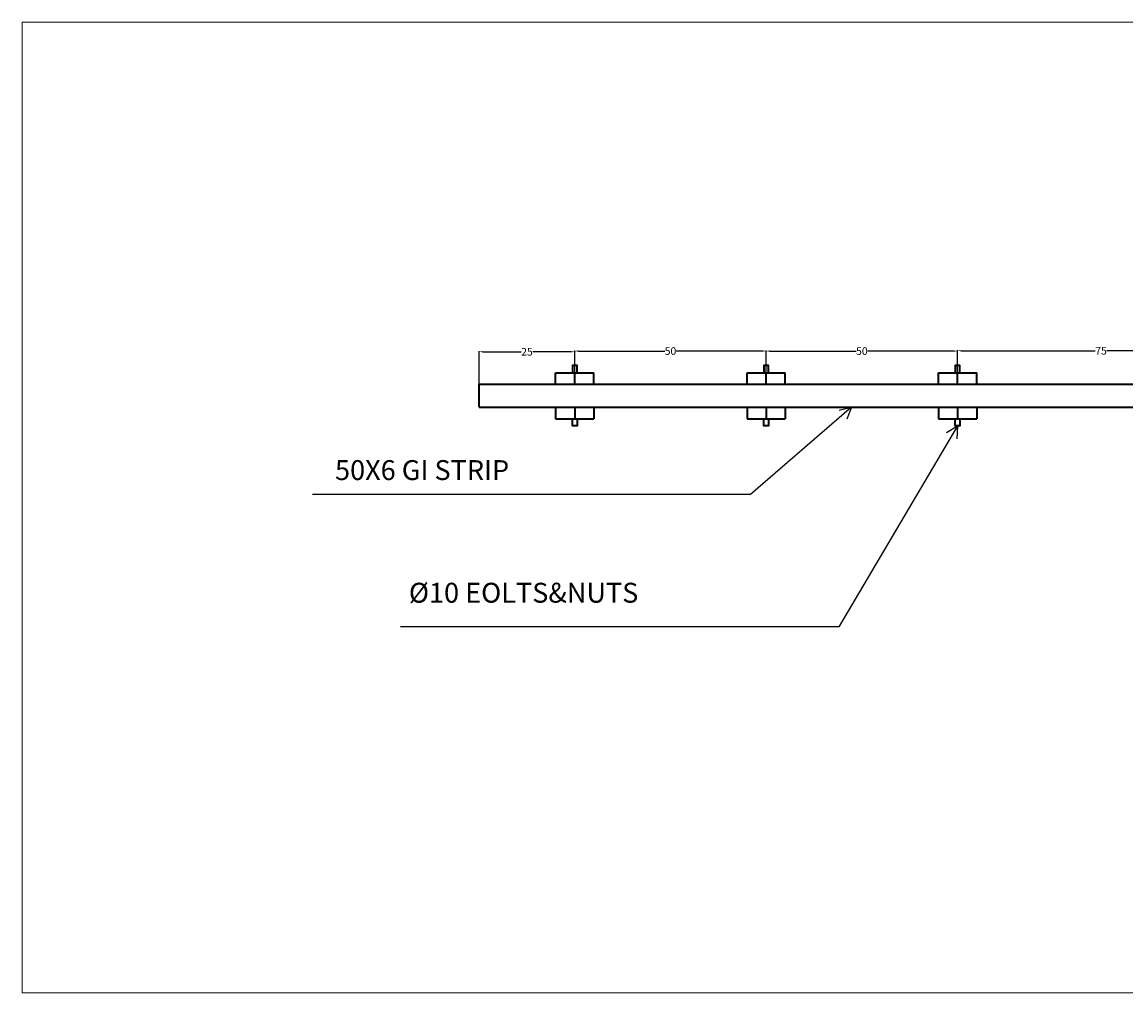
# Model space of a CAD drawing. Units: inches. Extents: x -129 to 2013, y -3652 to 814.
# Tile 2 of 5: x 98 to 387, y -1618 to -1364. Entities that reach past the tile are written whole.
import ezdxf

# ---------------------------------------------------------------- set-up
doc = ezdxf.new("R2010")
doc.units = ezdxf.units.IN
doc.header["$MEASUREMENT"] = 0
for name, color, linetype, lineweight in [('A-ANNO-DIMS', 2, 'Continuous', 18), ('A-ANNO-SYMB', 3, 'Continuous', 18), ('A-ANNO-TEXT', 7, 'Continuous', 25), ('E-GRND', 1, 'Continuous', 35)]:
    doc.layers.add(name, color=color, linetype=linetype, lineweight=lineweight)
doc.styles.get("Standard").update_dxf_attribs({"font": 'arial.ttf'})
doc.dimstyles.new('SMALL', dxfattribs={"dimtxt": 2, "dimasz": 1, "dimexe": 0.18, "dimexo": 0.0625, "dimgap": 0.09, "dimtad": 0, "dimdec": 0, "dimzin": 0, "dimdsep": 46, "dimtxsty": 'Standard', "dimcen": 0.09, "dimadec": 0, "dimazin": 0, "dimtfac": 1, "dimtdec": 0, "dimtofl": 0, "dimtmove": 0, "dimatfit": 3, "dimfxl": 1, "dimtolj": 1, "dimtzin": 0, "dimarcsym": 0})

# ---------------------------------------------------------------- blocks, each defined once
blk = doc.blocks.new('*D11')
at = {"layer": 'A-ANNO-DIMS', "color": 0, "lineweight": -2, "transparency": 16777216}
for p, q in [((217.51, -1458.55), (217.51, -1449.95)), ((218.51, -1450.13), (228.47, -1450.13)), ((241.51, -1450.13), (231.56, -1450.13)), ((242.51, -1458.55), (242.51, -1449.95))]:
    blk.add_line(p, q, dxfattribs=at)
at = {"layer": 'A-ANNO-DIMS', "color": 0, "transparency": 16777216}
for points in [[(218.51, -1449.96), (218.51, -1450.3), (217.51, -1450.13)], [(241.51, -1449.96), (241.51, -1450.3), (242.51, -1450.13)]]:
    blk.add_solid(points, dxfattribs=at)
at = {"layer": 'Defpoints', "color": 0, "transparency": 16777216}
for p in [(242.51, -1450.13), (217.51, -1458.61), (242.51, -1458.61)]:
    blk.add_point(p, dxfattribs=at)
at = {"layer": 'A-ANNO-DIMS', "color": 0, "transparency": 16777216, "insert": (230.01, -1450.13), "char_height": 2, "attachment_point": 5}
blk.add_mtext('\\A1;25', dxfattribs=at)
blk = doc.blocks.new('*D12')
at = {"layer": 'A-ANNO-DIMS', "color": 0, "lineweight": -2, "transparency": 16777216}
for p, q in [((242.51, -1458.55), (242.51, -1449.77)), ((243.51, -1449.95), (266, -1449.95)), ((291.51, -1449.95), (269.03, -1449.95)), ((292.51, -1458.55), (292.51, -1449.77))]:
    blk.add_line(p, q, dxfattribs=at)
at = {"layer": 'A-ANNO-DIMS', "color": 0, "transparency": 16777216}
for points in [[(243.51, -1449.78), (243.51, -1450.12), (242.51, -1449.95)], [(291.51, -1449.78), (291.51, -1450.12), (292.51, -1449.95)]]:
    blk.add_solid(points, dxfattribs=at)
at = {"layer": 'Defpoints', "color": 0, "transparency": 16777216}
for p in [(292.51, -1449.95), (242.51, -1458.61), (292.51, -1458.61)]:
    blk.add_point(p, dxfattribs=at)
at = {"layer": 'A-ANNO-DIMS', "color": 0, "transparency": 16777216, "insert": (267.51, -1449.95), "char_height": 2, "attachment_point": 5}
blk.add_mtext('\\A1;50', dxfattribs=at)
blk = doc.blocks.new('*D13')
at = {"layer": 'A-ANNO-DIMS', "color": 0, "lineweight": -2, "transparency": 16777216}
for p, q in [((292.51, -1458.55), (292.51, -1449.77)), ((293.51, -1449.95), (316, -1449.95)), ((341.51, -1449.95), (319.03, -1449.95)), ((342.51, -1458.55), (342.51, -1449.77))]:
    blk.add_line(p, q, dxfattribs=at)
at = {"layer": 'A-ANNO-DIMS', "color": 0, "transparency": 16777216}
for points in [[(293.51, -1449.78), (293.51, -1450.12), (292.51, -1449.95)], [(341.51, -1449.78), (341.51, -1450.12), (342.51, -1449.95)]]:
    blk.add_solid(points, dxfattribs=at)
at = {"layer": 'Defpoints', "color": 0, "transparency": 16777216}
for p in [(342.51, -1449.95), (292.51, -1458.61), (342.51, -1458.61)]:
    blk.add_point(p, dxfattribs=at)
at = {"layer": 'A-ANNO-DIMS', "color": 0, "transparency": 16777216, "insert": (317.51, -1449.95), "char_height": 2, "attachment_point": 5}
blk.add_mtext('\\A1;50', dxfattribs=at)
blk = doc.blocks.new('*D14')
at = {"layer": 'A-ANNO-DIMS', "color": 0, "lineweight": -2, "transparency": 16777216}
for p, q in [((342.51, -1458.55), (342.51, -1449.69)), ((343.51, -1449.87), (378.49, -1449.87)), ((416.51, -1449.87), (381.54, -1449.87)), ((417.51, -1458.55), (417.51, -1449.69))]:
    blk.add_line(p, q, dxfattribs=at)
at = {"layer": 'A-ANNO-DIMS', "color": 0, "transparency": 16777216}
for points in [[(343.51, -1449.7), (343.51, -1450.03), (342.51, -1449.87)], [(416.51, -1449.7), (416.51, -1450.03), (417.51, -1449.87)]]:
    blk.add_solid(points, dxfattribs=at)
at = {"layer": 'Defpoints', "color": 0, "transparency": 16777216}
for p in [(417.51, -1449.87), (342.51, -1458.61), (417.51, -1458.61)]:
    blk.add_point(p, dxfattribs=at)
at = {"layer": 'A-ANNO-DIMS', "color": 0, "transparency": 16777216, "insert": (380.01, -1449.87), "char_height": 2, "attachment_point": 5}
blk.add_mtext('\\A1;75', dxfattribs=at)
blk = doc.blocks.new('BOLT-M10')
for p, q in [((237.51, -1458.61), (237.51, -1455.61)), ((237.51, -1455.61), (247.51, -1455.61)), ((242.51, -1458.61), (242.51, -1455.61)), ((247.51, -1458.61), (247.51, -1455.61)), ((237.51, -1464.61), (237.51, -1467.61)), ((242.51, -1464.61), (242.51, -1467.61)), ((247.51, -1464.61), (247.51, -1467.61)), ((237.51, -1467.61), (247.51, -1467.61))]:
    blk.add_line(p, q)
for points in [[(241.89, -1455.61), (243.14, -1455.61), (243.14, -1453.74), (241.89, -1453.74)], [(241.89, -1467.61), (243.14, -1467.61), (243.14, -1469.49), (241.89, -1469.49)]]:
    blk.add_lwpolyline(points, close=True)

msp = doc.modelspace()

# ---------------------------------------------------------------- linework, layer by layer
at = {"layer": 'A-ANNO-SYMB'}
msp.add_lwpolyline([(674.9231, -1617.5657), (98.0927, -1617.5657), (98.0927, -1364.0415), (674.9231, -1364.0415)], close=True, dxfattribs=at)
at = {"layer": 'A-ANNO-TEXT'}
for points in [[(314.8334, -1464.6135), (288.4589, -1487.4409), (173.9784, -1487.4409)], [(311.5711, -1465.3903), (314.8334, -1464.6135), (313.5989, -1467.7316)], [(342.5146, -1469.4885), (311.4595, -1522.0022), (196.9789, -1522.0022)], [(339.6562, -1471.2423), (342.5146, -1469.4885), (342.3122, -1472.836)]]:
    msp.add_lwpolyline(points, dxfattribs=at)
at = {"layer": 'E-GRND'}
for p, q in [((217.5146, -1464.6135), (217.5146, -1458.6135)), ((217.5146, -1458.6135), (242.5146, -1458.6135)), ((242.5146, -1458.6135), (292.5146, -1458.6135)), ((292.5146, -1458.6135), (342.5146, -1458.6135)), ((342.5146, -1458.6135), (417.5146, -1458.6135)), ((217.5146, -1464.6135), (617.5146, -1464.6135)), ((242.5146, -1464.6135), (292.5146, -1464.6135)), ((292.5146, -1464.6135), (342.5146, -1464.6135)), ((342.5146, -1464.6135), (417.5146, -1464.6135))]:
    msp.add_line(p, q, dxfattribs=at)

# ---------------------------------------------------------------- block references
for p in [(0, 0), (50, 0), (100, 0)]:
    msp.add_blockref('BOLT-M10', p, dxfattribs=at)

# ---------------------------------------------------------------- texts
at = {"layer": 'A-ANNO-TEXT'}
msp.add_text('50X6 GI STRIP', height=5.191665, dxfattribs=at).set_placement((179.8623, -1483.6321))
at = {"layer": 'A-ANNO-TEXT', "insert": (199.1593, -1517.279), "char_height": 5.191665, "width": 83.281793, "attachment_point": 7}
msp.add_mtext('%%C10 EOLTS&NUTS', dxfattribs=at)

# ---------------------------------------------------------------- dimensions: what is measured, and where the dimension line sits
at = {"layer": 'A-ANNO-DIMS'}
for base, p1, p2, picture, middle in [((242.5146, -1450.1305), (217.5146, -1458.6135), (242.5146, -1458.6135), '*D11', (230.0146, -1450.1305)), ((292.5146, -1449.9505), (242.5146, -1458.6135), (292.5146, -1458.6135), '*D12', (267.5146, -1449.9505)), ((342.5146, -1449.9505), (292.5146, -1458.6135), (342.5146, -1458.6135), '*D13', (317.5146, -1449.9505)), ((417.5146, -1449.8672), (342.5146, -1458.6135), (417.5146, -1458.6135), '*D14', (380.0146, -1449.8672))]:
    dim = msp.add_linear_dim(base=base, p1=p1, p2=p2, dimstyle='SMALL', override={"dimclrd": 0, "dimclre": 0, "dimclrt": 0}, dxfattribs=at)
    dim.commit()
    dim.dimension.update_dxf_attribs({"geometry": picture, "text_midpoint": middle})

doc.saveas('drawing.dxf')
